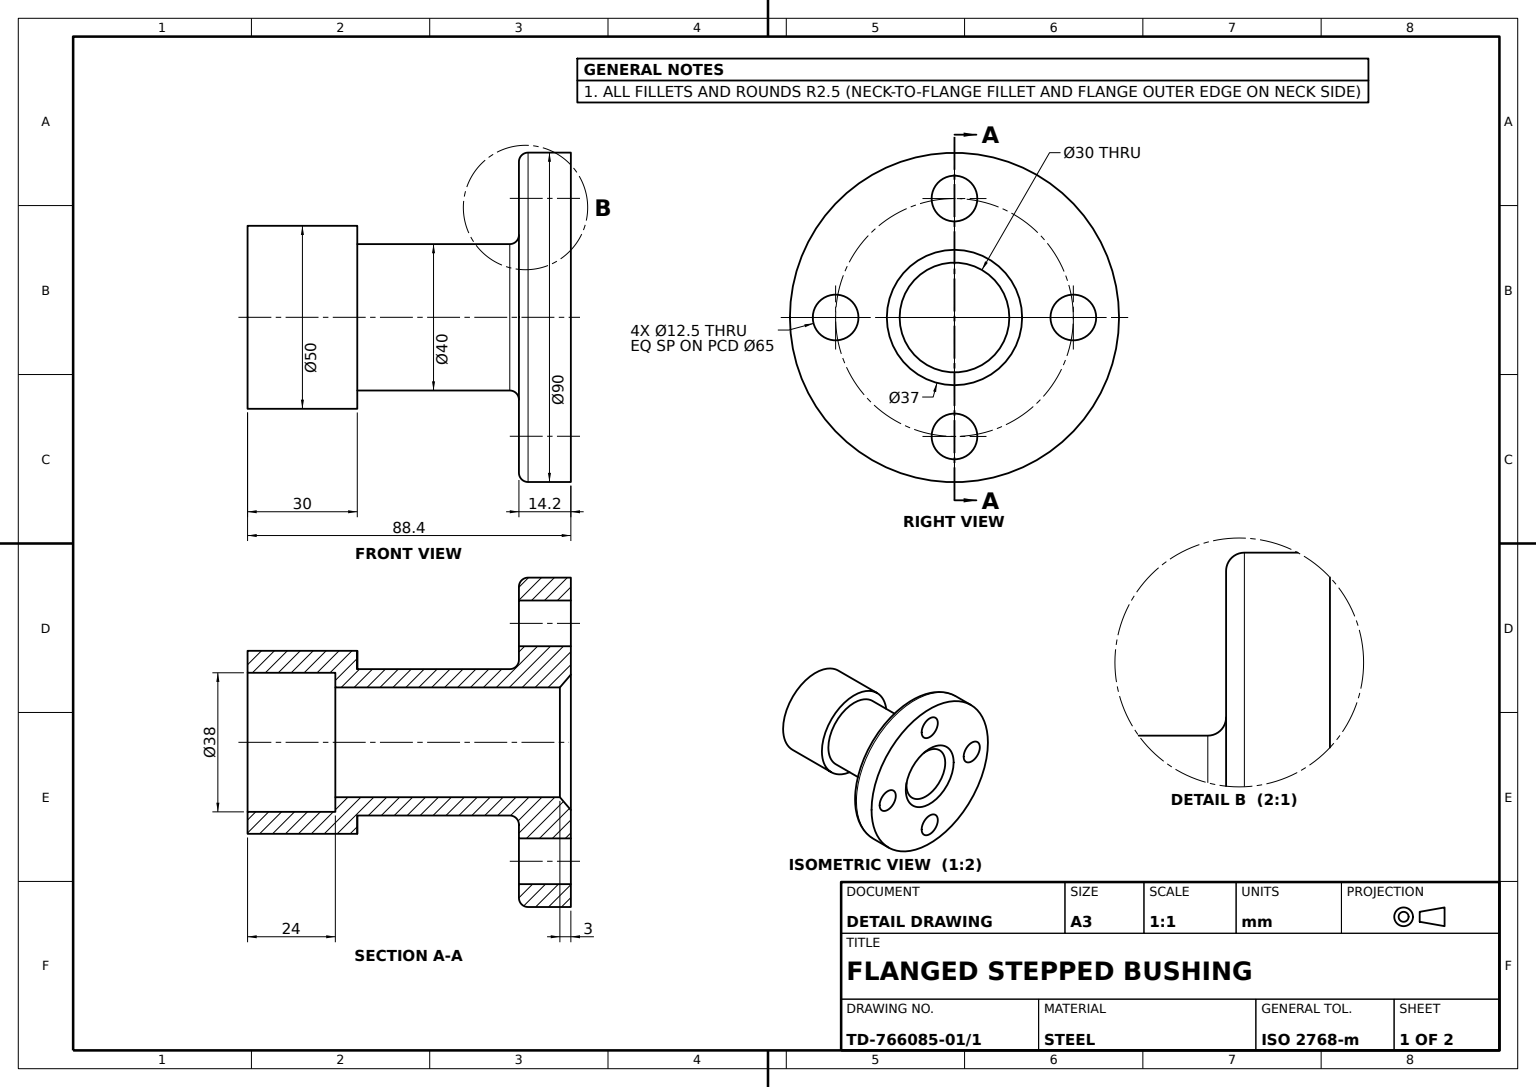
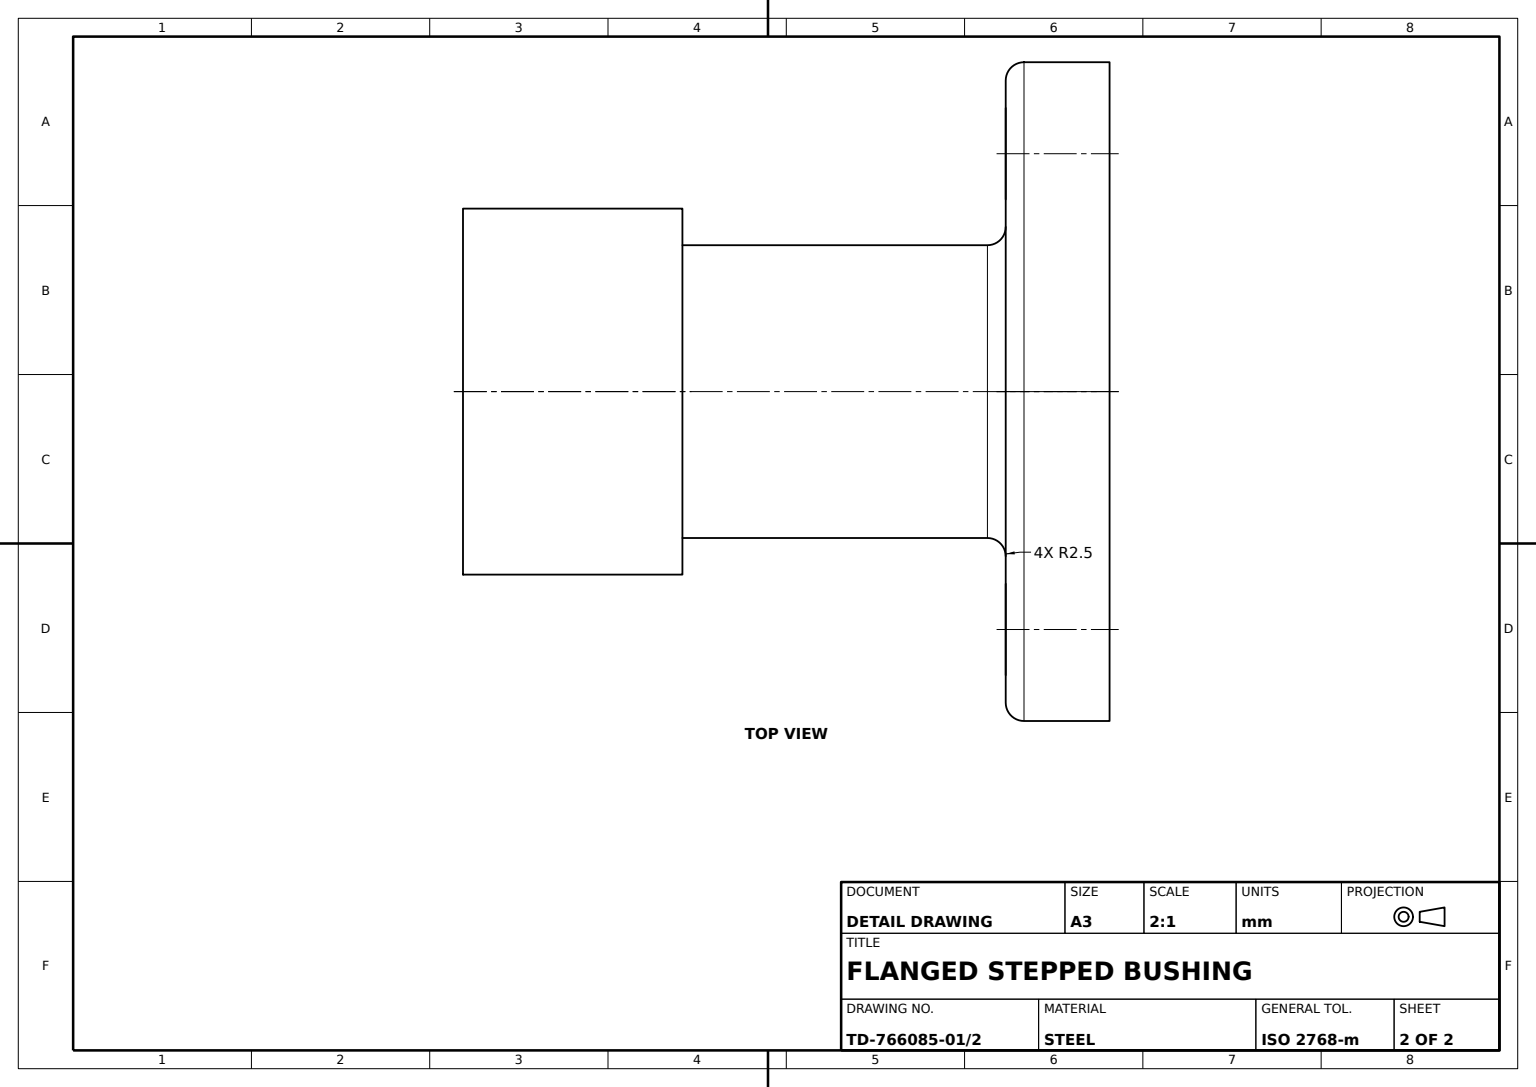
SolidWorks part; units mm, degrees
material "Plain Carbon Steel"
ref_plane "Front Plane" through (0, 0, 0) normal (0, 0, 1) x (1, 0, 0)
ref_plane "Top Plane" through (0, 0, 0) normal (0, 1, 0) x (1, 0, 0)
ref_plane "Right Plane" through (0, 0, 0) normal (1, 0, 0) x (0, 0, -1)
sketch "Flange Profile Sketch" plane through (0, 0, 0) normal (0, 0, 1) x (1, 0, 0)
  circle A0 centre (0, 0) radius 45
  circle A1 centre (0, 0) radius 15
  dimension "D1" = 90
  dimension "D2" = 30
extrude "Flange Ø90" add sketch "Flange Profile Sketch" along normal blind 14.2
sketch "Flange Holes Sketch" plane through (0, 0, 0) normal (0, 0, -1) x (-1, 0, 0)
  line L0 (-32.5, 0) -> (32.5, 0) construction
  line L1 (0, 32.5) -> (0, -32.5) construction
  circle A0 centre (-32.5, 0) radius 6.25
  circle A1 centre (32.5, 0) radius 6.25
  circle A2 centre (0, -32.5) radius 6.25
  circle A3 centre (0, 32.5) radius 6.25
  dimension "D3" = 12.5
  dimension "D4" = 12.5
  dimension "D7" = 12.5
  dimension "D8" = 12.5
  dimension "D1" = 65
  dimension "D2" = 32.5
  dimension "D5" = 65
  dimension "D6" = 32.5
extrude "Flange Holes 4xØ12.5" cut sketch "Flange Holes Sketch" against normal through all
chamfer "Flange Chamfer" distance 3 distance2 3.5 1 edges at (15, 0, 0)
sketch "Neck Profile Sketch" plane through (0, 0, 14.2) normal (0, 0, 1) x (1, 0, 0)
  circle A0 centre (0, 0) radius 15
  circle A1 centre (0, 0) radius 20
  dimension "D1" = 30
  dimension "D2" = 40
extrude "Neck Ø40" add sketch "Neck Profile Sketch" along normal blind 44.2 contours A1 | A0
fillet "Flange Edge Fillet R2.5" radius 2.5 1 edges at (45, 0, 14.2)
sketch "Collar Profile Sketch" plane through (0, 0, 58.4) normal (0, 0, 1) x (1, 0, 0)
  circle A0 centre (0, 0) radius 15
  circle A1 centre (0, 0) radius 25
  dimension "D1" = 30
  dimension "D2" = 50
extrude "Collar Ø50" add sketch "Collar Profile Sketch" along normal blind 6
sketch "End Sleeve Profile Sketch" plane through (0, 0, 64.4) normal (0, 0, 1) x (1, 0, 0)
  circle A0 centre (0, 0) radius 19
  circle A1 centre (0, 0) radius 25
  dimension "D1" = 38
  dimension "D2" = 50
extrude "End Sleeve Ø50 Bore Ø38" add sketch "End Sleeve Profile Sketch" along normal blind 24
fillet "Neck Root Fillet R2.5" radius 2.5 1 edges at (20, 0, 14.2)
